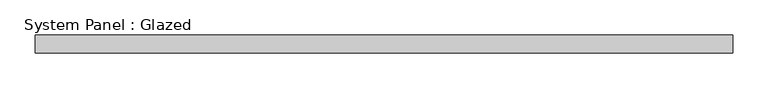
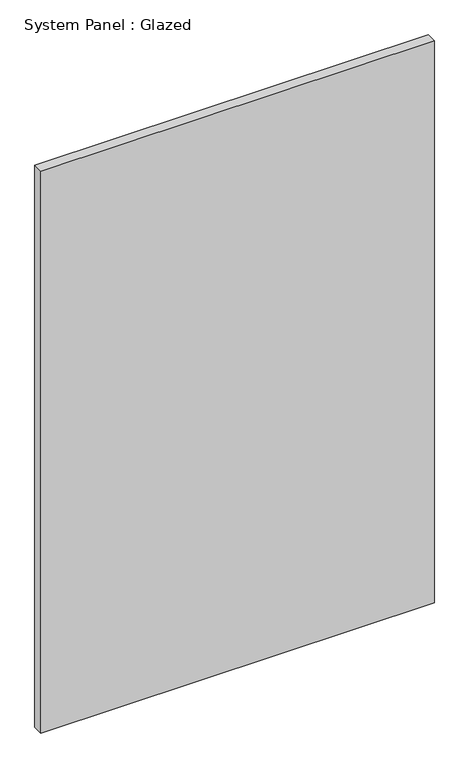
"""IFC4 building model written with IfcOpenShell, lengths in millimetres: plate geometry, System Panel : Glazed."""

from ifc_helpers import new_model, si_unit, origin, origin_with_axes, place, context, project, spatial, polyline, outline, extrude, source, transform, mapped, element, save


def system_panel_glazed_3519d5a1(model_context):
    return source(origin(), model_context, "Body", "SweptSolid", [
        extrude(outline(polyline([(495.3, 19.05), (-495.3, 19.05), (-495.3, 44.45), (495.3, 44.45), (495.3, 19.05)])), origin_with_axes(), (0.0, 0.0, 1.0), 1494.6448529),
    ])


if __name__ == "__main__":
    model = new_model("IFC4")
    model_context = context("Model", 3, world=origin())
    ifc_project = project(units=[si_unit("LENGTHUNIT", "METRE", prefix="MILLI")], contexts=[model_context])
    site = spatial("IfcSite", under=ifc_project)
    building = spatial("IfcBuilding", under=site)
    placement = place(None, origin())
    system_panel_glazed_shape = system_panel_glazed_3519d5a1(model_context)
    element("IfcPlate", 1, ObjectType="System Panel : Glazed", at=placement, inside=building, context=model_context, shape_type="MappedRepresentation", body=[
        mapped(system_panel_glazed_shape, transform((0.0, 0.0, 0.0), x_axis=(1.0, 0.0, 0.0), y_axis=(0.0, 1.0, 0.0), z_axis=(0.0, 0.0, 1.0))),
    ])
    save(model, "model.ifc")

# Revit data of these elements
# Type "System Panel : Glazed"
#   Construction Type Id = "GSP4R"
#   Analytic Construction = "1/8 in Pilkington single glazing"
#   Visual Light Transmittance = 0.9
#   Solar Heat Gain Coefficient = 0.86
#   Heat Transfer Coefficient (U) = 1.18115 BTU/(h·ft²·°F)
#   Define Thermal Properties by = 1
# Element 1 (IfcPlate, "System Panel : Glazed")
#   Materials on its faces: "Glass"
# Materials
#   "Glass": class "Glass", colour RGB 0 128 192, transparency 0.75, Description = "Soda Lime Glass", Cost = 0
